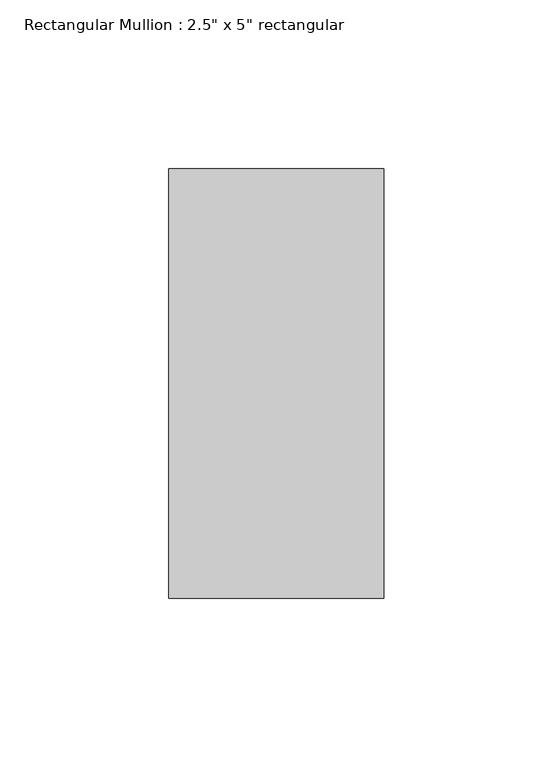
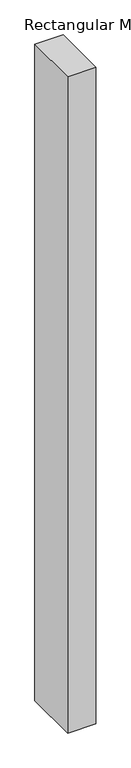
"""IFC4 building model written with IfcOpenShell, lengths in millimetres: member geometry."""

from ifc_helpers import new_model, si_unit, frame, origin, place, context, project, spatial, polyline, outline, extrude, source, transform, mapped, element, save


def member_76628514(model_context):
    return source(origin(), model_context, "Body", "SweptSolid", [
        extrude(outline(polyline([(31.75, 63.5), (31.75, -63.5), (-31.75, -63.5), (-31.75, 63.5), (31.75, 63.5)])), frame((0.0, 0.0, -1558.73195), z_axis=(0.0, 0.0, 1.0), x_axis=(1.0, 0.0, 0.0)), (0.0, 0.0, 1.0), 1558.73195),
    ])


if __name__ == "__main__":
    model = new_model("IFC4")
    model_context = context("Model", 3, world=origin())
    ifc_project = project(units=[si_unit("LENGTHUNIT", "METRE", prefix="MILLI")], contexts=[model_context])
    site = spatial("IfcSite", under=ifc_project)
    building = spatial("IfcBuilding", under=site)
    placement = place(None, origin())
    member_shape = member_76628514(model_context)
    element("IfcMember", 1, ObjectType="Rectangular Mullion : 2.5\" x 5\" rectangular", at=placement, inside=building, context=model_context, shape_type="MappedRepresentation", body=[
        mapped(member_shape, transform((0.0, 0.0, 0.0), x_axis=(1.0, 0.0, 0.0), y_axis=(0.0, 1.0, 0.0), z_axis=(0.0, 0.0, 1.0))),
    ])
    save(model, "model.ifc")

# Revit data of these elements
# Type "Rectangular Mullion : 2.5\" x 5\" rectangular"
#   built-in parameter 1007304 = 0.416667 (stored number, unit not read)
#   built-in parameter 1007301 = 0.104167 (stored number, unit not read)
#   built-in parameter 1007300 = 0.104167 (stored number, unit not read)
# Element 1 (IfcMember, "Rectangular Mullion : 2.5\" x 5\" rectangular")
#   Materials on its faces: "Aluminum"
# Materials
#   "Aluminum": class "Metal", colour RGB 247 247 247, transparency 0, Description = "Aluminum 6061", Cost = 0
